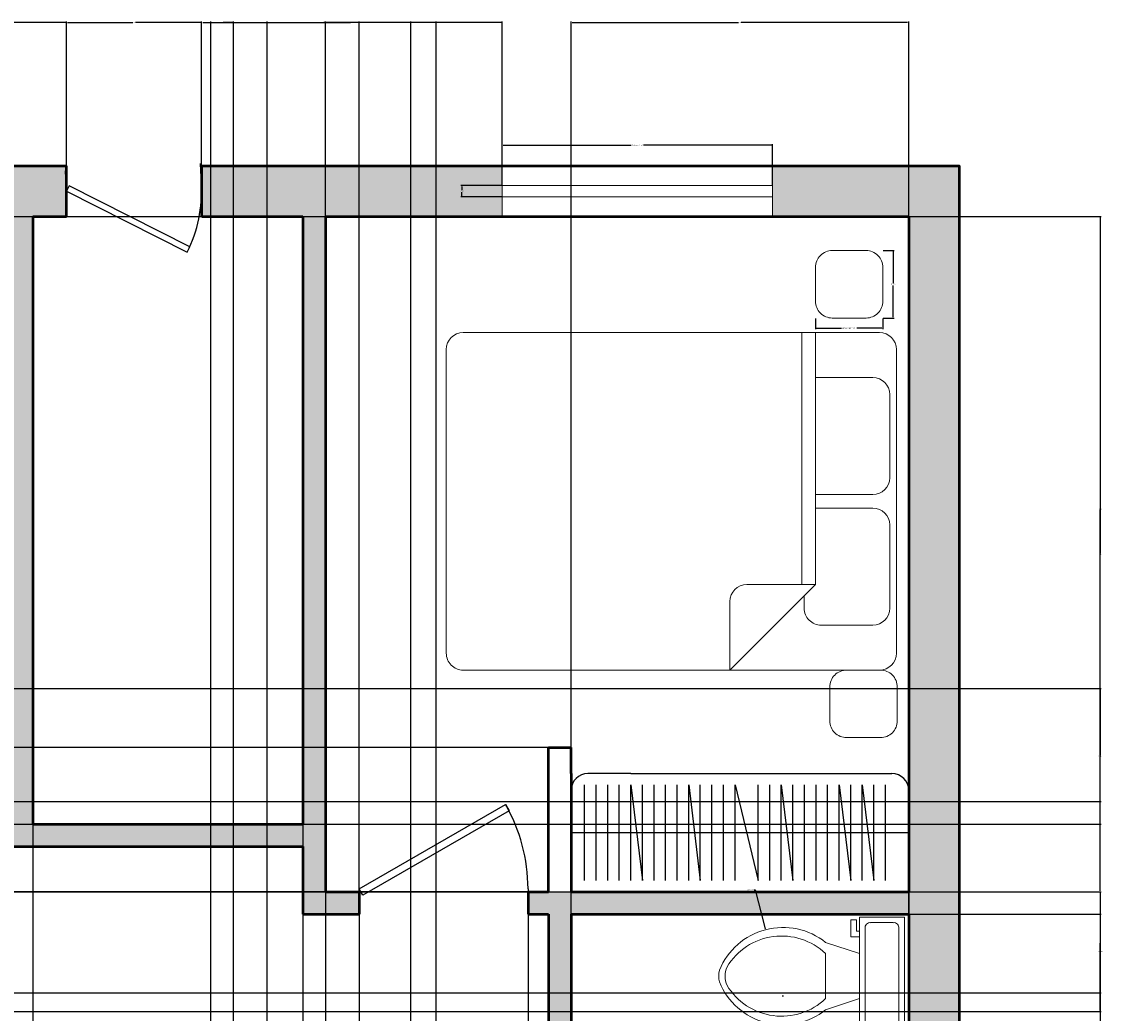
# Model space of a CAD drawing. Units: inches. Extents: x 3439 to 3988, y 1915 to 2284.
# Tile 7 of 7: x 3796 to 3988, y 2108 to 2284. Entities that reach past the tile are written whole.
import ezdxf

# ---------------------------------------------------------------- set-up
doc = ezdxf.new("R2010")
doc.units = ezdxf.units.IN
for name, color, linetype, lineweight in [('A-ANNO-DIMS', 2, 'Continuous', 18), ('A-DOOR', 3, 'Continuous', 25), ('A-FLOR-CASE', 8, 'Continuous', 25), ('A-FLOR-FIXT', 9, 'Continuous', 18), ('A-FURN', 9, 'Continuous', 18), ('A-GLAZ', 4, 'Continuous', 18), ('A-WALL', 7, 'Continuous', 50)]:
    doc.layers.add(name, color=color, linetype=linetype, lineweight=lineweight)
doc.layers.add('A-WALL-PATT', color=18, linetype='Continuous', lineweight=13, true_color=0x000000)
doc.styles.get("Standard").update_dxf_attribs({"font": 'arial.ttf'})
doc.dimstyles.get("Standard").update_dxf_attribs({"dimtxt": 0.18, "dimasz": 0.18, "dimexe": 0.18, "dimexo": 0.0625, "dimgap": 0.09, "dimtad": 0, "dimtih": 1, "dimtoh": 1, "dimdec": 4, "dimzin": 0, "dimdsep": 46, "dimtxsty": 'Standard', "dimcen": 0.09, "dimadec": 0, "dimazin": 0, "dimtfac": 1, "dimtdec": 4, "dimtofl": 0, "dimtmove": 0, "dimatfit": 3, "dimfxl": 1, "dimtolj": 1, "dimtzin": 0, "dimarcsym": 0})

# ---------------------------------------------------------------- blocks, each defined once
blk = doc.blocks.new('*U5')
for p, q in [((0, 0), (0, 6)), ((40, 0), (40, 6))]:
    blk.add_line(p, q)
blk.add_lwpolyline([(0, 0), (34.64, -20), (35.52, -18.48), (0.87, 1.52)], close=True)
blk.add_arc((0, 0), 40, 330, 0)
blk = doc.blocks.new('*U4')
for p, q in [((0, 0), (0, -6)), ((40, 0), (40, -6))]:
    blk.add_line(p, q)
blk.add_lwpolyline([(0, 0), (34.64, 20), (35.52, 18.48), (0.87, -1.52)], close=True)
blk.add_arc((0, 0), 40, 0, 30)
blk = doc.blocks.new('Toilet - top')
for p, q in [((9.5, -6), (9.5, -2)), ((-10, -8.5), (-8, -8.5)), ((-10, -9.5), (-10, -8.5)), ((-7, -9.5), (-10, -9.5)), ((-8, -8.5), (-8, -8)), ((-7, -8), (-7, -9.5)), ((-4, -8), (-6, -14)), ((4, -8), (6, -14)), ((4, -14), (-4, -14))]:
    blk.add_line(p, q)
blk.add_lwpolyline([(10.5, -8), (10.5, 0), (-10.5, 0), (-10.5, -8)], close=True)
for points in [[(8.5, -1), (-8.5, -1)], [(-9.5, -2), (-9.5, -6)], [(-8.5, -7), (8.5, -7)]]:
    blk.add_lwpolyline(points)
for centre, radius, start, end in [((-8.62, -1.88), 0.884, 81.8699, 188.1301), ((8.62, -1.88), 0.884, 351.8699, 98.1301), ((-8.62, -6.12), 0.884, 171.8699, 278.1301), ((8.62, -6.12), 0.884, 261.8699, 8.1301), ((3.52, -21.58), 12.17, 141.4691, 247.9714), ((4.2, -21.82), 11.33, 136.3677, 238.9468), ((-3.52, -21.58), 12.17, 292.0284, 38.5307), ((-4.2, -21.82), 11.33, 301.053, 43.6321), ((0, -27.88), 4, 245.7318, 294.2682), ((0, -29), 4, 254.8605, 285.1395)]:
    blk.add_arc(centre, radius, start, end)
blk = doc.blocks.new('Bed - Queen')
for p, q in [((3, 0), (56.99999, 0)), ((10.99999, -1.2), (25.79998, -1.2)), ((34.19999, -1.2), (48.99999, -1.2)), ((0, -77.00003), (0, -3)), ((59.99999, -3), (59.99999, -77.00003)), ((7.99999, -14.4), (7.99999, -4.2)), ((28.79998, -4.2), (28.79998, -14.4)), ((31.19999, -14.4), (31.19999, -4.2)), ((51.99999, -4.2), (51.99999, -13.4)), ((0, -14.4), (44.8, -14.4)), ((59.99999, -29.6), (44.8, -14.4)), ((44.8, -14.4), (44.8, -26.6)), ((44.8, -16.8), (0, -16.8)), ((48.99999, -16.4), (46.79936, -16.4)), ((47.8, -29.6), (59.99999, -29.6)), ((56.99999, -80.00003), (3, -80.00003))]:
    blk.add_line(p, q)
for centre, start, end in [((3, -3), 90, 180), ((56.99999, -3), 0, 90), ((10.99999, -4.2), 90, 180), ((25.79998, -4.2), 0, 90), ((34.19999, -4.2), 90, 180), ((48.99999, -4.2), 0, 90), ((48.99999, -13.4), 270, 0), ((47.8, -26.6), 180, 270), ((3, -77.00003), 180, 270), ((56.99999, -77.00003), 270, 0)]:
    blk.add_arc(centre, 3, start, end)
blk = doc.blocks.new('WINDOW-GLASS-48IN')
for p, q in [((0, 2), (48, 2)), ((0, 0), (48, 0))]:
    blk.add_line(p, q)
blk = doc.blocks.new('NIGHTSTAND-12IN-RADIUS')
blk.add_lwpolyline([(3, 0), (9, 0, 0.414214), (12, 3), (12, 9, 0.414214), (9, 12), (3, 12, 0.414214), (0, 9), (0, 3, 0.414214)], format="xyb", close=True)
blk = doc.blocks.new('*D19')
at = {"layer": 'A-ANNO-DIMS', "color": 0, "lineweight": -2, "transparency": 16777216}
for p, q in [((3881.36, 2254.92), (3881.36, 2262.24)), ((3881.54, 2262.06), (3904.24, 2262.06)), ((3929.18, 2262.06), (3906.47, 2262.06)), ((3929.36, 2254.92), (3929.36, 2262.24))]:
    blk.add_line(p, q, dxfattribs=at)
at = {"layer": 'A-ANNO-DIMS', "color": 0, "transparency": 16777216}
for points in [[(3881.54, 2262.09), (3881.54, 2262.03), (3881.36, 2262.06)], [(3929.18, 2262.09), (3929.18, 2262.03), (3929.36, 2262.06)]]:
    blk.add_solid(points, dxfattribs=at)
at = {"layer": 'Defpoints', "color": 0, "transparency": 16777216}
for p in [(3929.36, 2262.06), (3881.36, 2254.86), (3929.36, 2254.86)]:
    blk.add_point(p, dxfattribs=at)
at = {"layer": 'A-ANNO-DIMS', "color": 0, "transparency": 16777216, "insert": (3905.36, 2262.06), "char_height": 0.18, "attachment_point": 5}
blk.add_mtext('\\A1;WINDOW 48 TYP.', dxfattribs=at)
blk = doc.blocks.new('*D20')
at = {"layer": 'A-ANNO-DIMS', "color": 0, "lineweight": -2, "transparency": 16777216}
for p, q in [((3881.29, 2254.86), (3873.98, 2254.86)), ((3874.16, 2254.68), (3874.16, 2254.04)), ((3874.16, 2253.04), (3874.16, 2253.68)), ((3881.29, 2252.86), (3873.98, 2252.86))]:
    blk.add_line(p, q, dxfattribs=at)
at = {"layer": 'A-ANNO-DIMS', "color": 0, "transparency": 16777216}
for points in [[(3874.13, 2254.68), (3874.19, 2254.68), (3874.16, 2254.86)], [(3874.13, 2253.04), (3874.19, 2253.04), (3874.16, 2252.86)]]:
    blk.add_solid(points, dxfattribs=at)
at = {"layer": 'Defpoints', "color": 0, "transparency": 16777216}
for p in [(3874.16, 2254.86), (3881.36, 2254.86), (3881.36, 2252.86)]:
    blk.add_point(p, dxfattribs=at)
at = {"layer": 'A-ANNO-DIMS', "color": 0, "transparency": 16777216, "insert": (3874.16, 2253.86), "char_height": 0.18, "attachment_point": 5}
blk.add_mtext('\\A1;2 TYP.', dxfattribs=at)
blk = doc.blocks.new('*D27')
at = {"layer": 'A-ANNO-DIMS', "color": 0, "lineweight": -2, "transparency": 16777216}
for p, q in [((3937, 2231.25), (3937, 2229.33)), ((3949, 2231.25), (3949, 2229.33)), ((3937.18, 2229.51), (3941.63, 2229.51)), ((3948.82, 2229.51), (3944.38, 2229.51))]:
    blk.add_line(p, q, dxfattribs=at)
at = {"layer": 'A-ANNO-DIMS', "color": 0, "transparency": 16777216}
for points in [[(3937.18, 2229.54), (3937.18, 2229.48), (3937, 2229.51)], [(3948.82, 2229.54), (3948.82, 2229.48), (3949, 2229.51)]]:
    blk.add_solid(points, dxfattribs=at)
at = {"layer": 'Defpoints', "color": 0, "transparency": 16777216}
for p in [(3937, 2231.31), (3949, 2231.31), (3949, 2229.51)]:
    blk.add_point(p, dxfattribs=at)
at = {"layer": 'A-ANNO-DIMS', "color": 0, "transparency": 16777216, "insert": (3943, 2229.51), "char_height": 0.18, "attachment_point": 5}
blk.add_mtext('\\A1;NIGHTSTAND 12 TYP.', dxfattribs=at)
blk = doc.blocks.new('*D28')
at = {"layer": 'A-ANNO-DIMS', "color": 0, "lineweight": -2, "transparency": 16777216}
for p, q in [((3949.07, 2243.31), (3950.98, 2243.31)), ((3950.8, 2243.13), (3950.8, 2237.49)), ((3950.8, 2231.49), (3950.8, 2237.13)), ((3949.07, 2231.31), (3950.98, 2231.31))]:
    blk.add_line(p, q, dxfattribs=at)
at = {"layer": 'A-ANNO-DIMS', "color": 0, "transparency": 16777216}
for points in [[(3950.77, 2243.13), (3950.83, 2243.13), (3950.8, 2243.31)], [(3950.77, 2231.49), (3950.83, 2231.49), (3950.8, 2231.31)]]:
    blk.add_solid(points, dxfattribs=at)
at = {"layer": 'Defpoints', "color": 0, "transparency": 16777216}
for p in [(3949, 2243.31), (3950.8, 2243.31), (3949, 2231.31)]:
    blk.add_point(p, dxfattribs=at)
at = {"layer": 'A-ANNO-DIMS', "color": 0, "transparency": 16777216, "insert": (3950.8, 2237.31), "char_height": 0.18, "attachment_point": 5}
blk.add_mtext('\\A1;12 TYP.', dxfattribs=at)
blk = doc.blocks.new('*D50')
at = {"layer": 'A-ANNO-DIMS', "color": 0, "lineweight": -2, "transparency": 16777216}
for p, q in [((3797.93, 2249.3), (3797.93, 1915.13)), ((3845.93, 2249.3), (3845.93, 1915.13)), ((3798.11, 1915.31), (3821.71, 1915.31)), ((3845.75, 1915.31), (3822.15, 1915.31))]:
    blk.add_line(p, q, dxfattribs=at)
at = {"layer": 'A-ANNO-DIMS', "color": 0, "transparency": 16777216}
for points in [[(3798.11, 1915.34), (3798.11, 1915.28), (3797.93, 1915.31)], [(3845.75, 1915.34), (3845.75, 1915.28), (3845.93, 1915.31)]]:
    blk.add_solid(points, dxfattribs=at)
at = {"layer": 'Defpoints', "color": 0, "transparency": 16777216}
for p in [(3797.93, 2249.36), (3845.93, 2249.36), (3845.93, 1915.31)]:
    blk.add_point(p, dxfattribs=at)
at = {"layer": 'A-ANNO-DIMS', "color": 0, "transparency": 16777216, "insert": (3821.93, 1915.31), "char_height": 0.18, "attachment_point": 5}
blk.add_mtext('\\A1;48', dxfattribs=at)
blk = doc.blocks.new('*D51')
at = {"layer": 'A-ANNO-DIMS', "color": 0, "lineweight": -2, "transparency": 16777216}
for p, q in [((3849.93, 2249.3), (3849.93, 1915.13)), ((3953.58, 2249.3), (3953.58, 1915.13)), ((3850.11, 1915.31), (3901.3, 1915.31)), ((3953.4, 1915.31), (3902.21, 1915.31))]:
    blk.add_line(p, q, dxfattribs=at)
at = {"layer": 'A-ANNO-DIMS', "color": 0, "transparency": 16777216}
for points in [[(3850.11, 1915.34), (3850.11, 1915.28), (3849.93, 1915.31)], [(3953.4, 1915.34), (3953.4, 1915.28), (3953.58, 1915.31)]]:
    blk.add_solid(points, dxfattribs=at)
at = {"layer": 'Defpoints', "color": 0, "transparency": 16777216}
for p in [(3849.93, 2249.36), (3953.58, 2249.36), (3953.58, 1915.31)]:
    blk.add_point(p, dxfattribs=at)
at = {"layer": 'A-ANNO-DIMS', "color": 0, "transparency": 16777216, "insert": (3901.76, 1915.31), "char_height": 0.18, "attachment_point": 5}
blk.add_mtext('\\A1;103.65', dxfattribs=at)
blk = doc.blocks.new('*D58')
at = {"layer": 'A-ANNO-DIMS', "color": 0, "lineweight": -2, "transparency": 16777216}
for p, q in [((3953.64, 2249.36), (3987.81, 2249.36)), ((3987.63, 2249.18), (3987.63, 2189.54)), ((3987.63, 2129.54), (3987.63, 2189.18)), ((3953.64, 2129.36), (3987.81, 2129.36))]:
    blk.add_line(p, q, dxfattribs=at)
at = {"layer": 'A-ANNO-DIMS', "color": 0, "transparency": 16777216}
for points in [[(3987.6, 2249.18), (3987.66, 2249.18), (3987.63, 2249.36)], [(3987.6, 2129.54), (3987.66, 2129.54), (3987.63, 2129.36)]]:
    blk.add_solid(points, dxfattribs=at)
at = {"layer": 'Defpoints', "color": 0, "transparency": 16777216}
for p in [(3953.58, 2249.36), (3987.63, 2249.36), (3953.58, 2129.36)]:
    blk.add_point(p, dxfattribs=at)
at = {"layer": 'A-ANNO-DIMS', "color": 0, "transparency": 16777216, "insert": (3987.63, 2189.36), "char_height": 0.18, "attachment_point": 5}
blk.add_mtext('\\A1;120', dxfattribs=at)
blk = doc.blocks.new('*D59')
at = {"layer": 'A-ANNO-DIMS', "color": 0, "lineweight": -2, "transparency": 16777216}
for p, q in [((3953.64, 2125.36), (3987.81, 2125.36)), ((3987.63, 2125.18), (3987.63, 2095.54)), ((3987.63, 2065.54), (3987.63, 2095.18)), ((3953.64, 2065.36), (3987.81, 2065.36))]:
    blk.add_line(p, q, dxfattribs=at)
at = {"layer": 'A-ANNO-DIMS', "color": 0, "transparency": 16777216}
for points in [[(3987.6, 2125.18), (3987.66, 2125.18), (3987.63, 2125.36)], [(3987.6, 2065.54), (3987.66, 2065.54), (3987.63, 2065.36)]]:
    blk.add_solid(points, dxfattribs=at)
at = {"layer": 'Defpoints', "color": 0, "transparency": 16777216}
for p in [(3953.58, 2125.36), (3987.63, 2125.36), (3953.58, 2065.36)]:
    blk.add_point(p, dxfattribs=at)
at = {"layer": 'A-ANNO-DIMS', "color": 0, "transparency": 16777216, "insert": (3987.63, 2095.36), "char_height": 0.18, "attachment_point": 5}
blk.add_mtext('\\A1;60', dxfattribs=at)
blk = doc.blocks.new('*D63')
at = {"layer": 'A-ANNO-DIMS', "color": 0, "lineweight": -2, "transparency": 16777216}
for p, q in [((3893.58, 2065.42), (3893.58, 2284)), ((3893.76, 2283.82), (3923.36, 2283.82)), ((3953.4, 2283.82), (3923.8, 2283.82)), ((3953.58, 2065.42), (3953.58, 2284))]:
    blk.add_line(p, q, dxfattribs=at)
at = {"layer": 'A-ANNO-DIMS', "color": 0, "transparency": 16777216}
for points in [[(3893.76, 2283.85), (3893.76, 2283.79), (3893.58, 2283.82)], [(3953.4, 2283.85), (3953.4, 2283.79), (3953.58, 2283.82)]]:
    blk.add_solid(points, dxfattribs=at)
at = {"layer": 'Defpoints', "color": 0, "transparency": 16777216}
for p in [(3953.58, 2283.82), (3893.58, 2065.36), (3953.58, 2065.36)]:
    blk.add_point(p, dxfattribs=at)
at = {"layer": 'A-ANNO-DIMS', "color": 0, "transparency": 16777216, "insert": (3923.58, 2283.82), "char_height": 0.18, "attachment_point": 5}
blk.add_mtext('\\A1;60', dxfattribs=at)
blk = doc.blocks.new('*D64')
at = {"layer": 'A-ANNO-DIMS', "color": 0, "lineweight": -2, "transparency": 16777216}
for p, q in [((3593.64, 2249.36), (3987.81, 2249.36)), ((3987.63, 2249.18), (3987.63, 2197.54)), ((3987.63, 2145.54), (3987.63, 2197.18)), ((3593.64, 2145.36), (3987.81, 2145.36))]:
    blk.add_line(p, q, dxfattribs=at)
at = {"layer": 'A-ANNO-DIMS', "color": 0, "transparency": 16777216}
for points in [[(3987.6, 2249.18), (3987.66, 2249.18), (3987.63, 2249.36)], [(3987.6, 2145.54), (3987.66, 2145.54), (3987.63, 2145.36)]]:
    blk.add_solid(points, dxfattribs=at)
at = {"layer": 'Defpoints', "color": 0, "transparency": 16777216}
for p in [(3593.58, 2249.36), (3987.63, 2249.36), (3593.58, 2145.36)]:
    blk.add_point(p, dxfattribs=at)
at = {"layer": 'A-ANNO-DIMS', "color": 0, "transparency": 16777216, "insert": (3987.63, 2197.36), "char_height": 0.18, "attachment_point": 5}
blk.add_mtext('\\A1;104', dxfattribs=at)
blk = doc.blocks.new('*D65')
at = {"layer": 'A-ANNO-DIMS', "color": 0, "lineweight": -2, "transparency": 16777216}
for p, q in [((3797.99, 2249.36), (3987.81, 2249.36)), ((3987.63, 2249.18), (3987.63, 2195.54)), ((3987.63, 2141.54), (3987.63, 2195.18)), ((3797.99, 2141.36), (3987.81, 2141.36))]:
    blk.add_line(p, q, dxfattribs=at)
at = {"layer": 'A-ANNO-DIMS', "color": 0, "transparency": 16777216}
for points in [[(3987.6, 2249.18), (3987.66, 2249.18), (3987.63, 2249.36)], [(3987.6, 2141.54), (3987.66, 2141.54), (3987.63, 2141.36)]]:
    blk.add_solid(points, dxfattribs=at)
at = {"layer": 'Defpoints', "color": 0, "transparency": 16777216}
for p in [(3797.93, 2249.36), (3987.63, 2249.36), (3797.93, 2141.36)]:
    blk.add_point(p, dxfattribs=at)
at = {"layer": 'A-ANNO-DIMS', "color": 0, "transparency": 16777216, "insert": (3987.63, 2195.36), "char_height": 0.18, "attachment_point": 5}
blk.add_mtext('\\A1;108', dxfattribs=at)
blk = doc.blocks.new('*D69')
at = {"layer": 'A-ANNO-DIMS', "color": 0, "lineweight": -2, "transparency": 16777216}
for p, q in [((3739.41, 2258.42), (3739.41, 2284)), ((3739.59, 2283.82), (3771.27, 2283.82)), ((3803.75, 2283.82), (3772.06, 2283.82)), ((3803.93, 2258.42), (3803.93, 2284))]:
    blk.add_line(p, q, dxfattribs=at)
at = {"layer": 'A-ANNO-DIMS', "color": 0, "transparency": 16777216}
for points in [[(3739.59, 2283.85), (3739.59, 2283.79), (3739.41, 2283.82)], [(3803.75, 2283.85), (3803.75, 2283.79), (3803.93, 2283.82)]]:
    blk.add_solid(points, dxfattribs=at)
at = {"layer": 'Defpoints', "color": 0, "transparency": 16777216}
for p in [(3803.93, 2283.82), (3739.41, 2258.36), (3803.93, 2258.36)]:
    blk.add_point(p, dxfattribs=at)
at = {"layer": 'A-ANNO-DIMS', "color": 0, "transparency": 16777216, "insert": (3771.67, 2283.82), "char_height": 0.18, "attachment_point": 5}
blk.add_mtext('\\A1;64.53', dxfattribs=at)
blk = doc.blocks.new('*D70')
at = {"layer": 'A-ANNO-DIMS', "color": 0, "lineweight": -2, "transparency": 16777216}
for p, q in [((3803.93, 2258.42), (3803.93, 2284)), ((3804.11, 2283.82), (3815.71, 2283.82)), ((3827.75, 2283.82), (3816.15, 2283.82)), ((3827.93, 2258.42), (3827.93, 2284))]:
    blk.add_line(p, q, dxfattribs=at)
at = {"layer": 'A-ANNO-DIMS', "color": 0, "transparency": 16777216}
for points in [[(3804.11, 2283.85), (3804.11, 2283.79), (3803.93, 2283.82)], [(3827.75, 2283.85), (3827.75, 2283.79), (3827.93, 2283.82)]]:
    blk.add_solid(points, dxfattribs=at)
at = {"layer": 'Defpoints', "color": 0, "transparency": 16777216}
for p in [(3827.93, 2283.82), (3803.93, 2258.36), (3827.93, 2258.36)]:
    blk.add_point(p, dxfattribs=at)
at = {"layer": 'A-ANNO-DIMS', "color": 0, "transparency": 16777216, "insert": (3815.93, 2283.82), "char_height": 0.18, "attachment_point": 5}
blk.add_mtext('\\A1;24', dxfattribs=at)
blk = doc.blocks.new('*D71')
at = {"layer": 'A-ANNO-DIMS', "color": 0, "lineweight": -2, "transparency": 16777216}
for p, q in [((3827.93, 2258.42), (3827.93, 2284)), ((3828.11, 2283.82), (3854.25, 2283.82)), ((3881.18, 2283.82), (3855.04, 2283.82)), ((3881.36, 2258.42), (3881.36, 2284))]:
    blk.add_line(p, q, dxfattribs=at)
at = {"layer": 'A-ANNO-DIMS', "color": 0, "transparency": 16777216}
for points in [[(3828.11, 2283.85), (3828.11, 2283.79), (3827.93, 2283.82)], [(3881.18, 2283.85), (3881.18, 2283.79), (3881.36, 2283.82)]]:
    blk.add_solid(points, dxfattribs=at)
at = {"layer": 'Defpoints', "color": 0, "transparency": 16777216}
for p in [(3881.36, 2283.82), (3827.93, 2258.36), (3881.36, 2258.36)]:
    blk.add_point(p, dxfattribs=at)
at = {"layer": 'A-ANNO-DIMS', "color": 0, "transparency": 16777216, "insert": (3854.64, 2283.82), "char_height": 0.18, "attachment_point": 5}
blk.add_mtext('\\A1;53.42', dxfattribs=at)
blk = doc.blocks.new('*D76')
at = {"layer": 'A-ANNO-DIMS', "color": 0, "lineweight": -2, "transparency": 16777216}
for p, q in [((3833.58, 1949.42), (3833.58, 2284)), ((3833.76, 2283.82), (3849.01, 2283.82)), ((3864.9, 2283.82), (3849.66, 2283.82)), ((3865.08, 1949.42), (3865.08, 2284))]:
    blk.add_line(p, q, dxfattribs=at)
at = {"layer": 'A-ANNO-DIMS', "color": 0, "transparency": 16777216}
for points in [[(3833.76, 2283.85), (3833.76, 2283.79), (3833.58, 2283.82)], [(3864.9, 2283.85), (3864.9, 2283.79), (3865.08, 2283.82)]]:
    blk.add_solid(points, dxfattribs=at)
at = {"layer": 'Defpoints', "color": 0, "transparency": 16777216}
for p in [(3865.08, 2283.82), (3833.58, 1949.36), (3865.08, 1949.36)]:
    blk.add_point(p, dxfattribs=at)
at = {"layer": 'A-ANNO-DIMS', "color": 0, "transparency": 16777216, "insert": (3849.33, 2283.82), "char_height": 0.18, "attachment_point": 5}
blk.add_mtext('\\A1;31.5', dxfattribs=at)
blk = doc.blocks.new('*D77')
at = {"layer": 'A-ANNO-DIMS', "color": 0, "lineweight": -2, "transparency": 16777216}
for p, q in [((3473.64, 2129.36), (3987.81, 2129.36)), ((3987.63, 2129.18), (3987.63, 2118.9)), ((3987.63, 2108.25), (3987.63, 2118.53)), ((3473.64, 2108.07), (3987.81, 2108.07))]:
    blk.add_line(p, q, dxfattribs=at)
at = {"layer": 'A-ANNO-DIMS', "color": 0, "transparency": 16777216}
for points in [[(3987.6, 2129.18), (3987.66, 2129.18), (3987.63, 2129.36)], [(3987.6, 2108.25), (3987.66, 2108.25), (3987.63, 2108.07)]]:
    blk.add_solid(points, dxfattribs=at)
at = {"layer": 'Defpoints', "color": 0, "transparency": 16777216}
for p in [(3473.58, 2129.36), (3987.63, 2129.36), (3473.58, 2108.07)]:
    blk.add_point(p, dxfattribs=at)
at = {"layer": 'A-ANNO-DIMS', "color": 0, "transparency": 16777216, "insert": (3987.63, 2118.71), "char_height": 0.18, "attachment_point": 5}
blk.add_mtext('\\A1;21.295', dxfattribs=at)
blk = doc.blocks.new('*D82')
at = {"layer": 'A-ANNO-DIMS', "color": 0, "lineweight": -2, "transparency": 16777216}
for p, q in [((3537.64, 2129.36), (3987.81, 2129.36)), ((3987.63, 2129.18), (3987.63, 2120.54)), ((3987.63, 2111.54), (3987.63, 2120.18)), ((3537.64, 2111.36), (3987.81, 2111.36))]:
    blk.add_line(p, q, dxfattribs=at)
at = {"layer": 'A-ANNO-DIMS', "color": 0, "transparency": 16777216}
for points in [[(3987.6, 2129.18), (3987.66, 2129.18), (3987.63, 2129.36)], [(3987.6, 2111.54), (3987.66, 2111.54), (3987.63, 2111.36)]]:
    blk.add_solid(points, dxfattribs=at)
at = {"layer": 'Defpoints', "color": 0, "transparency": 16777216}
for p in [(3537.58, 2129.36), (3987.63, 2129.36), (3537.58, 2111.36)]:
    blk.add_point(p, dxfattribs=at)
at = {"layer": 'A-ANNO-DIMS', "color": 0, "transparency": 16777216, "insert": (3987.63, 2120.36), "char_height": 0.18, "attachment_point": 5}
blk.add_mtext('\\A1;18', dxfattribs=at)
blk = doc.blocks.new('*D83')
at = {"layer": 'A-ANNO-DIMS', "color": 0, "lineweight": -2, "transparency": 16777216}
for p, q in [((3537.64, 2111.36), (3987.81, 2111.36)), ((3987.63, 2111.18), (3987.63, 2099.54)), ((3987.63, 2087.54), (3987.63, 2099.18)), ((3537.64, 2087.36), (3987.81, 2087.36))]:
    blk.add_line(p, q, dxfattribs=at)
at = {"layer": 'A-ANNO-DIMS', "color": 0, "transparency": 16777216}
for points in [[(3987.6, 2111.18), (3987.66, 2111.18), (3987.63, 2111.36)], [(3987.6, 2087.54), (3987.66, 2087.54), (3987.63, 2087.36)]]:
    blk.add_solid(points, dxfattribs=at)
at = {"layer": 'Defpoints', "color": 0, "transparency": 16777216}
for p in [(3537.58, 2111.36), (3987.63, 2111.36), (3537.58, 2087.36)]:
    blk.add_point(p, dxfattribs=at)
at = {"layer": 'A-ANNO-DIMS', "color": 0, "transparency": 16777216, "insert": (3987.63, 2099.36), "char_height": 0.18, "attachment_point": 5}
blk.add_mtext('\\A1;24', dxfattribs=at)
blk = doc.blocks.new('*D84')
at = {"layer": 'A-ANNO-DIMS', "color": 0, "lineweight": -2, "transparency": 16777216}
for p, q in [((3849.93, 2129.42), (3849.93, 2284)), ((3850.11, 2283.82), (3852.78, 2283.82)), ((3855.75, 2283.82), (3853.08, 2283.82)), ((3855.93, 2129.42), (3855.93, 2284))]:
    blk.add_line(p, q, dxfattribs=at)
at = {"layer": 'A-ANNO-DIMS', "color": 0, "transparency": 16777216}
for points in [[(3850.11, 2283.85), (3850.11, 2283.79), (3849.93, 2283.82)], [(3855.75, 2283.85), (3855.75, 2283.79), (3855.93, 2283.82)]]:
    blk.add_solid(points, dxfattribs=at)
at = {"layer": 'Defpoints', "color": 0, "transparency": 16777216}
for p in [(3855.93, 2283.82), (3849.93, 2129.36), (3855.93, 2129.36)]:
    blk.add_point(p, dxfattribs=at)
at = {"layer": 'A-ANNO-DIMS', "color": 0, "transparency": 16777216, "insert": (3852.93, 2283.82), "char_height": 0.18, "attachment_point": 5}
blk.add_mtext('\\A1;6', dxfattribs=at)
blk = doc.blocks.new('*D85')
at = {"layer": 'A-ANNO-DIMS', "color": 0, "lineweight": -2, "transparency": 16777216}
for p, q in [((3855.93, 2125.3), (3855.93, 1915.13)), ((3885.93, 2125.3), (3885.93, 1915.13)), ((3856.11, 1915.31), (3870.71, 1915.31)), ((3885.75, 1915.31), (3871.15, 1915.31))]:
    blk.add_line(p, q, dxfattribs=at)
at = {"layer": 'A-ANNO-DIMS', "color": 0, "transparency": 16777216}
for points in [[(3856.11, 1915.34), (3856.11, 1915.28), (3855.93, 1915.31)], [(3885.75, 1915.34), (3885.75, 1915.28), (3885.93, 1915.31)]]:
    blk.add_solid(points, dxfattribs=at)
at = {"layer": 'Defpoints', "color": 0, "transparency": 16777216}
for p in [(3855.93, 2125.36), (3885.93, 2125.36), (3885.93, 1915.31)]:
    blk.add_point(p, dxfattribs=at)
at = {"layer": 'A-ANNO-DIMS', "color": 0, "transparency": 16777216, "insert": (3870.93, 1915.31), "char_height": 0.18, "attachment_point": 5}
blk.add_mtext('\\A1;30', dxfattribs=at)
blk = doc.blocks.new('*D87')
at = {"layer": 'A-ANNO-DIMS', "color": 0, "lineweight": -2, "transparency": 16777216}
for p, q in [((3839.58, 2065.42), (3839.58, 2284)), ((3839.76, 2283.82), (3854.36, 2283.82)), ((3869.4, 2283.82), (3854.8, 2283.82)), ((3869.58, 2065.42), (3869.58, 2284))]:
    blk.add_line(p, q, dxfattribs=at)
at = {"layer": 'A-ANNO-DIMS', "color": 0, "transparency": 16777216}
for points in [[(3839.76, 2283.85), (3839.76, 2283.79), (3839.58, 2283.82)], [(3869.4, 2283.85), (3869.4, 2283.79), (3869.58, 2283.82)]]:
    blk.add_solid(points, dxfattribs=at)
at = {"layer": 'Defpoints', "color": 0, "transparency": 16777216}
for p in [(3869.58, 2283.82), (3839.58, 2065.36), (3869.58, 2065.36)]:
    blk.add_point(p, dxfattribs=at)
at = {"layer": 'A-ANNO-DIMS', "color": 0, "transparency": 16777216, "insert": (3854.58, 2283.82), "char_height": 0.18, "attachment_point": 5}
blk.add_mtext('\\A1;30', dxfattribs=at)
blk = doc.blocks.new('*D93')
at = {"layer": 'A-ANNO-DIMS', "color": 0, "lineweight": -2, "transparency": 16777216}
for p, q in [((3829.58, 2065.42), (3829.58, 2284)), ((3829.76, 2283.82), (3831.43, 2283.82)), ((3833.4, 2283.82), (3831.73, 2283.82)), ((3833.58, 2061.42), (3833.58, 2284))]:
    blk.add_line(p, q, dxfattribs=at)
at = {"layer": 'A-ANNO-DIMS', "color": 0, "transparency": 16777216}
for points in [[(3829.76, 2283.85), (3829.76, 2283.79), (3829.58, 2283.82)], [(3833.4, 2283.85), (3833.4, 2283.79), (3833.58, 2283.82)]]:
    blk.add_solid(points, dxfattribs=at)
at = {"layer": 'Defpoints', "color": 0, "transparency": 16777216}
for p in [(3833.58, 2283.82), (3829.58, 2065.36), (3833.58, 2061.36)]:
    blk.add_point(p, dxfattribs=at)
at = {"layer": 'A-ANNO-DIMS', "color": 0, "transparency": 16777216, "insert": (3831.58, 2283.82), "char_height": 0.18, "attachment_point": 5}
blk.add_mtext('\\A1;4', dxfattribs=at)
blk = doc.blocks.new('*D95')
at = {"layer": 'A-ANNO-DIMS', "color": 0, "lineweight": -2, "transparency": 16777216}
for p, q in [((3729.47, 2165.5), (3987.81, 2165.5)), ((3987.63, 2165.32), (3987.63, 2153.61)), ((3987.63, 2141.54), (3987.63, 2153.25)), ((3729.47, 2141.36), (3987.81, 2141.36))]:
    blk.add_line(p, q, dxfattribs=at)
at = {"layer": 'A-ANNO-DIMS', "color": 0, "transparency": 16777216}
for points in [[(3987.6, 2165.32), (3987.66, 2165.32), (3987.63, 2165.5)], [(3987.6, 2141.54), (3987.66, 2141.54), (3987.63, 2141.36)]]:
    blk.add_solid(points, dxfattribs=at)
at = {"layer": 'Defpoints', "color": 0, "transparency": 16777216}
for p in [(3729.41, 2165.5), (3987.63, 2165.5), (3729.41, 2141.36)]:
    blk.add_point(p, dxfattribs=at)
at = {"layer": 'A-ANNO-DIMS', "color": 0, "transparency": 16777216, "insert": (3987.63, 2153.43), "char_height": 0.18, "attachment_point": 5}
blk.add_mtext('\\A1;24.14', dxfattribs=at)
blk = doc.blocks.new('*D98')
at = {"layer": 'A-ANNO-DIMS', "color": 0, "lineweight": -2, "transparency": 16777216}
for p, q in [((3889.52, 2154.99), (3439.35, 2154.99)), ((3439.53, 2154.81), (3439.53, 2142.36)), ((3439.53, 2129.54), (3439.53, 2141.99)), ((3889.52, 2129.36), (3439.35, 2129.36))]:
    blk.add_line(p, q, dxfattribs=at)
at = {"layer": 'A-ANNO-DIMS', "color": 0, "transparency": 16777216}
for points in [[(3439.5, 2154.81), (3439.56, 2154.81), (3439.53, 2154.99)], [(3439.5, 2129.54), (3439.56, 2129.54), (3439.53, 2129.36)]]:
    blk.add_solid(points, dxfattribs=at)
at = {"layer": 'Defpoints', "color": 0, "transparency": 16777216}
for p in [(3889.58, 2154.99), (3439.53, 2129.36), (3889.58, 2129.36)]:
    blk.add_point(p, dxfattribs=at)
at = {"layer": 'A-ANNO-DIMS', "color": 0, "transparency": 16777216, "insert": (3439.53, 2142.18), "char_height": 0.18, "attachment_point": 5}
blk.add_mtext('\\A1;25.63', dxfattribs=at)
blk = doc.blocks.new('*D103')
at = {"layer": 'A-ANNO-DIMS', "color": 0, "lineweight": -2, "transparency": 16777216}
for p, q in [((3926.12, 2129.67), (3926.3, 2129.67)), ((3926.3, 2129.67), (3928.1, 2122.78)), ((3931.24, 2110.74), (3931.24, 2110.92)), ((3931.15, 2110.83), (3931.33, 2110.83))]:
    blk.add_line(p, q, dxfattribs=at)
at = {"layer": 'A-ANNO-DIMS', "color": 0, "transparency": 16777216}
blk.add_solid([(3928.13, 2122.79), (3928.08, 2122.77), (3928.15, 2122.6)], dxfattribs=at)
at = {"layer": 'Defpoints', "color": 0, "transparency": 16777216}
for p in [(3928.15, 2122.6), (3931.24, 2110.83)]:
    blk.add_point(p, dxfattribs=at)
at = {"layer": 'A-ANNO-DIMS', "color": 0, "transparency": 16777216, "insert": (3925.44, 2129.67), "char_height": 0.18, "attachment_point": 5}
blk.add_mtext('\\A1;6X R12.17', dxfattribs=at)

msp = doc.modelspace()

# ---------------------------------------------------------------- hatches: boundary and pattern name
at = {"layer": 'A-WALL-PATT'}
h = msp.add_hatch(color=256, dxfattribs=at)
h.dxf.hatch_style = 1
h.paths.add_polyline_path([(3803.9319, 2258.3617), (3739.4053, 2258.3617), (3739.4053, 2249.3617), (3793.9319, 2249.3617), (3793.9319, 2137.3617), (3845.9319, 2137.3617), (3845.9319, 2125.3617), (3855.9319, 2125.3617), (3855.9319, 2129.3617), (3849.9319, 2129.3617), (3849.9319, 2249.3617), (3881.3564, 2249.3617), (3881.3564, 2258.3617), (3827.9319, 2258.3617), (3827.9319, 2249.3617), (3845.9319, 2249.3617), (3845.9319, 2141.3617), (3797.9319, 2141.3617), (3797.9319, 2249.3617), (3803.9319, 2249.3617)])
h = msp.add_hatch(color=256, dxfattribs=at)
h.dxf.hatch_style = 1
h.paths.add_polyline_path([(3962.5815, 2258.3617), (3929.3564, 2258.3617), (3929.3564, 2249.3617), (3953.5815, 2249.3617), (3953.5815, 2129.3617), (3885.9319, 2129.3617), (3885.9319, 2125.3617), (3889.5815, 2125.3617), (3889.5815, 2095.3617), (3893.5815, 2095.3617), (3893.5815, 2125.3617), (3953.5815, 2125.3617), (3953.5815, 2065.3617), (3893.5815, 2065.3617), (3893.5815, 2071.3617), (3889.5815, 2071.3617), (3889.5815, 2065.3617), (3869.5815, 2065.3617), (3869.5815, 2061.3617), (3953.5815, 2061.3617), (3953.5815, 1949.3617), (3913.0815, 1949.3617), (3913.0815, 1940.3617), (3962.5815, 1940.3617)])

# ---------------------------------------------------------------- linework, layer by layer
at = {"layer": 'A-FLOR-CASE'}
for p, q in [((3904.206, 2150.3617), (3896.5815, 2150.3617)), ((3904.206, 2150.3617), (3950.5815, 2150.3617)), ((3904.206, 2150.3617), (3950.5815, 2150.3617)), ((3953.5815, 2150.3617), (3953.5815, 2129.3617)), ((3895.9789, 2131.3617), (3895.9789, 2148.3617)), ((3895.9789, 2131.3617), (3895.9789, 2148.3617)), ((3898.0357, 2131.3617), (3898.0357, 2148.3617)), ((3898.0357, 2131.3617), (3898.0357, 2148.3617)), ((3900.0924, 2131.3617), (3900.0924, 2148.3617)), ((3900.0924, 2131.3617), (3900.0924, 2148.3617)), ((3902.1492, 2131.3617), (3902.1492, 2148.3617)), ((3902.1492, 2131.3617), (3902.1492, 2148.3617)), ((3904.206, 2131.3617), (3904.206, 2148.3617)), ((3904.206, 2148.3617), (3906.2627, 2131.3617)), ((3904.206, 2131.3617), (3904.206, 2148.3617)), ((3904.206, 2148.3617), (3906.2627, 2131.3617)), ((3906.2627, 2131.3617), (3906.2627, 2148.3617)), ((3906.2627, 2131.3617), (3906.2627, 2148.3617)), ((3906.2627, 2131.3617), (3906.2627, 2148.3617)), ((3906.2627, 2131.3617), (3906.2627, 2148.3617)), ((3908.3195, 2131.3617), (3908.3195, 2148.3617)), ((3908.3195, 2131.3617), (3908.3195, 2148.3617)), ((3910.3763, 2131.3617), (3910.3763, 2148.3617)), ((3910.3763, 2131.3617), (3910.3763, 2148.3617)), ((3912.4331, 2131.3617), (3912.4331, 2148.3617)), ((3912.4331, 2131.3617), (3912.4331, 2148.3617)), ((3914.4898, 2131.3617), (3914.4898, 2148.3617)), ((3914.4898, 2148.3617), (3916.5466, 2131.3617)), ((3914.4898, 2131.3617), (3914.4898, 2148.3617)), ((3914.4898, 2148.3617), (3916.5466, 2131.3617)), ((3916.5466, 2131.3617), (3916.5466, 2148.3617)), ((3916.5466, 2131.3617), (3916.5466, 2148.3617)), ((3918.6034, 2131.3617), (3918.6034, 2148.3617)), ((3918.6034, 2131.3617), (3918.6034, 2148.3617)), ((3920.6601, 2131.3617), (3920.6601, 2148.3617)), ((3920.6601, 2131.3617), (3920.6601, 2148.3617)), ((3922.7169, 2131.3617), (3922.7169, 2148.3617)), ((3922.7169, 2148.3617), (3926.8305, 2131.3617)), ((3922.7169, 2131.3617), (3922.7169, 2148.3617)), ((3922.7169, 2148.3617), (3926.8305, 2131.3617)), ((3926.8305, 2131.3617), (3926.8305, 2148.3617)), ((3926.8305, 2131.3617), (3926.8305, 2148.3617)), ((3928.8872, 2131.3617), (3928.8872, 2148.3617)), ((3928.8872, 2131.3617), (3928.8872, 2148.3617)), ((3930.944, 2131.3617), (3930.944, 2148.3617)), ((3930.944, 2148.3617), (3933.0008, 2131.3617)), ((3930.944, 2131.3617), (3930.944, 2148.3617)), ((3930.944, 2148.3617), (3933.0008, 2131.3617)), ((3933.0008, 2131.3617), (3933.0008, 2148.3617)), ((3933.0008, 2131.3617), (3933.0008, 2148.3617)), ((3935.0575, 2131.3617), (3935.0575, 2148.3617)), ((3935.0575, 2131.3617), (3935.0575, 2148.3617)), ((3937.1143, 2131.3617), (3937.1143, 2148.3617)), ((3937.1143, 2131.3617), (3937.1143, 2148.3617)), ((3939.1711, 2131.3617), (3939.1711, 2148.3617)), ((3939.1711, 2131.3617), (3939.1711, 2148.3617)), ((3941.2278, 2131.3617), (3941.2278, 2148.3617)), ((3941.2278, 2148.3617), (3943.2846, 2131.3617)), ((3941.2278, 2131.3617), (3941.2278, 2148.3617)), ((3941.2278, 2148.3617), (3943.2846, 2131.3617)), ((3943.2846, 2131.3617), (3943.2846, 2148.3617)), ((3943.2846, 2131.3617), (3943.2846, 2148.3617)), ((3945.3414, 2131.3617), (3945.3414, 2148.3617)), ((3945.3414, 2148.3617), (3947.3982, 2131.3617)), ((3945.3414, 2131.3617), (3945.3414, 2148.3617)), ((3945.3414, 2148.3617), (3947.3982, 2131.3617)), ((3947.3982, 2131.3617), (3947.3982, 2148.3617)), ((3947.3982, 2131.3617), (3947.3982, 2148.3617)), ((3949.4549, 2131.3617), (3949.4549, 2148.3617)), ((3949.4549, 2131.3617), (3949.4549, 2148.3617)), ((3893.5815, 2147.3617), (3893.5815, 2129.3617)), ((3953.5815, 2147.3617), (3953.5815, 2129.3617)), ((3893.9221, 2139.8617), (3943.2976, 2139.8617)), ((3893.9221, 2139.8617), (3943.2976, 2139.8617)), ((3904.206, 2139.8617), (3953.5815, 2139.8617)), ((3904.206, 2139.8617), (3953.5815, 2139.8617)), ((3904.206, 2129.3617), (3893.5815, 2129.3617)), ((3953.5815, 2129.3617), (3904.206, 2129.3617)), ((3953.5815, 2129.3617), (3904.206, 2129.3617))]:
    msp.add_line(p, q, dxfattribs=at)
for centre, start, end in [((3896.5815, 2147.3617), 90, 180), ((3950.5815, 2147.3617), 0, 90), ((3950.5815, 2147.3617), 0, 90)]:
    msp.add_arc(centre, 3, start, end, dxfattribs=at)
at = {"layer": 'A-GLAZ'}
for points in [[(3881.3564, 2249.3617), (3881.3564, 2258.3617)], [(3929.3564, 2258.3617), (3929.3564, 2249.3617)]]:
    msp.add_lwpolyline(points, dxfattribs=at)
at = {"layer": 'A-WALL'}
for p, q in [((3803.9319, 2249.3617), (3803.9319, 2258.3617)), ((3827.9319, 2249.3617), (3827.9319, 2258.3617)), ((3797.9319, 2249.3617), (3797.9319, 2141.3617)), ((3797.9319, 2249.3617), (3803.9319, 2249.3617)), ((3827.9319, 2249.3617), (3845.9319, 2249.3617)), ((3833.5815, 2249.3617), (3845.9319, 2249.3617)), ((3845.9319, 2249.3617), (3845.9319, 2141.3617)), ((3849.9319, 2249.3617), (3849.9319, 2129.3617)), ((3849.9319, 2249.3617), (3953.5815, 2249.3617)), ((3953.5815, 2249.3617), (3953.5815, 2129.3617)), ((3889.5815, 2129.3617), (3889.5815, 2154.9906)), ((3889.5815, 2154.9906), (3893.5815, 2154.9906)), ((3893.5815, 2150.3617), (3893.5815, 2154.9906)), ((3893.5815, 2150.3617), (3893.5815, 2129.3617)), ((3797.9319, 2141.3617), (3845.9319, 2141.3617)), ((3793.9319, 2137.3617), (3845.9319, 2137.3617)), ((3845.9319, 2137.3617), (3845.9319, 2125.3617)), ((3849.9319, 2129.3617), (3855.9319, 2129.3617)), ((3855.9319, 2129.3617), (3855.9319, 2125.3617)), ((3885.9319, 2129.3617), (3885.9319, 2125.3617)), ((3885.9319, 2129.3617), (3889.5815, 2129.3617)), ((3893.5815, 2129.3617), (3953.5815, 2129.3617)), ((3845.9319, 2125.3617), (3855.9319, 2125.3617)), ((3885.9319, 2125.3617), (3889.5815, 2125.3617)), ((3889.5815, 2125.3617), (3889.5815, 2095.3617)), ((3893.5815, 2125.3617), (3893.5815, 2095.3617)), ((3893.5815, 2125.3617), (3953.5815, 2125.3617)), ((3953.5815, 2125.3617), (3953.5815, 2065.3617))]:
    msp.add_line(p, q, dxfattribs=at)
for points in [[(3719.5815, 1940.3617), (3464.5815, 1940.3617), (3464.5815, 2258.3617), (3803.9319, 2258.3617)], [(3827.9319, 2258.3617), (3962.5815, 2258.3617), (3962.5815, 1940.3617), (3767.5815, 1940.3617)]]:
    msp.add_lwpolyline(points, dxfattribs=at)

# ---------------------------------------------------------------- block references
at = {"layer": 'A-DOOR', "xscale": 0.5999999999999996, "yscale": 0.5999999999999996, "zscale": 0.5999999999999996, "rotation": 3.144592659610589}
msp.add_blockref('*U5', (3803.9319, 2253.8617), dxfattribs=at)
at = {"layer": 'A-DOOR', "xscale": 0.75, "yscale": 0.75, "zscale": 0.75}
msp.add_blockref('*U4', (3855.9319, 2129.8617), dxfattribs=at)
at = {"layer": 'A-FLOR-FIXT', "rotation": 269.9999999999999}
msp.add_blockref('Toilet - top', (3952.8222, 2114.3538), dxfattribs=at)
at = {"layer": 'A-FURN'}
for p in [(3937.0047, 2231.3134), (3939.5603, 2156.7366)]:
    msp.add_blockref('NIGHTSTAND-12IN-RADIUS', p, dxfattribs=at)
at = {"layer": 'A-FURN', "rotation": 270}
msp.add_blockref('Bed - Queen', (3951.4053, 2228.7366), dxfattribs=at)
at = {"layer": 'A-GLAZ'}
msp.add_blockref('WINDOW-GLASS-48IN', (3881.3564, 2252.8617), dxfattribs=at)

# ---------------------------------------------------------------- dimensions: what is measured, and where the dimension line sits
at = {"layer": 'A-ANNO-DIMS'}
for base, p1, p2, override, picture, middle in [((3803.9319, 2283.8228), (3739.4053, 2258.3617), (3803.9319, 2258.3617), {"dimdec": 2, "dimlfac": 1, "dimrnd": 0, "dimzin": 0, "dimdsep": 46, "dimlunit": 2}, '*D69', (3771.6686, 2283.8228)), ((3827.9319, 2283.8228), (3803.9319, 2258.3617), (3827.9319, 2258.3617), {"dimdec": 0, "dimlfac": 1, "dimrnd": 0, "dimzin": 0, "dimdsep": 46, "dimlunit": 2}, '*D70', (3815.9319, 2283.8228)), ((3881.3564, 2283.8228), (3827.9319, 2258.3617), (3881.3564, 2258.3617), {"dimdec": 2, "dimlfac": 1, "dimrnd": 0, "dimzin": 0, "dimdsep": 46, "dimlunit": 2}, '*D71', (3854.6442, 2283.8228)), ((3833.5815, 2283.8228), (3829.5815, 2065.3617), (3833.5815, 2061.3617), {"dimdec": 0, "dimlfac": 1, "dimrnd": 0, "dimzin": 0, "dimdsep": 46, "dimlunit": 2}, '*D93', (3831.5815, 2283.8228)), ((3865.0815, 2283.8228), (3833.5815, 1949.3617), (3865.0815, 1949.3617), {"dimdec": 1, "dimlfac": 1, "dimrnd": 0, "dimzin": 0, "dimdsep": 46, "dimlunit": 2}, '*D76', (3849.3315, 2283.8228)), ((3869.5815, 2283.8228), (3839.5815, 2065.3617), (3869.5815, 2065.3617), {"dimdec": 0, "dimlfac": 1, "dimrnd": 0, "dimzin": 0, "dimdsep": 46, "dimlunit": 2}, '*D87', (3854.5815, 2283.8228)), ((3855.9319, 2283.8228), (3849.9319, 2129.3617), (3855.9319, 2129.3617), {"dimdec": 0, "dimlfac": 1, "dimrnd": 0, "dimzin": 0, "dimdsep": 46, "dimlunit": 2}, '*D84', (3852.9319, 2283.8228)), ((3953.5815, 2283.8228), (3893.5815, 2065.3617), (3953.5815, 2065.3617), {"dimdec": 0, "dimlfac": 1, "dimrnd": 0, "dimzin": 0, "dimdsep": 46, "dimlunit": 2}, '*D63', (3923.5815, 2283.8228)), ((3845.9319, 1915.3117), (3797.9319, 2249.3617), (3845.9319, 2249.3617), {"dimdec": 0, "dimlfac": 1, "dimrnd": 0, "dimzin": 0, "dimdsep": 46, "dimlunit": 2}, '*D50', (3821.9319, 1915.3117)), ((3953.5815, 1915.3117), (3849.9319, 2249.3617), (3953.5815, 2249.3617), {"dimdec": 2, "dimlfac": 1, "dimrnd": 0, "dimzin": 0, "dimdsep": 46, "dimlunit": 2}, '*D51', (3901.7567, 1915.3117)), ((3885.9319, 1915.3117), (3855.9319, 2125.3617), (3885.9319, 2125.3617), {"dimdec": 0, "dimlfac": 1, "dimrnd": 0, "dimzin": 0, "dimdsep": 46, "dimlunit": 2}, '*D85', (3870.9319, 1915.3117))]:
    dim = msp.add_linear_dim(base=base, p1=p1, p2=p2, dimstyle='Standard', override=override, dxfattribs=at)
    dim.commit()
    dim.dimension.update_dxf_attribs({"geometry": picture, "text_midpoint": middle})
for base, p1, p2, text, picture, middle in [((3929.3564, 2262.0617), (3881.3564, 2254.8617), (3929.3564, 2254.8617), 'WINDOW <> TYP.', '*D19', (3905.3564, 2262.0617)), ((3949.0047, 2229.5134), (3937.0047, 2231.3134), (3949.0047, 2231.3134), 'NIGHTSTAND <> TYP.', '*D27', (3943.0047, 2229.5134))]:
    dim = msp.add_linear_dim(base=base, p1=p1, p2=p2, text=text, dimstyle='Standard', override={"dimdec": 0, "dimlfac": 1, "dimrnd": 0, "dimzin": 0, "dimdsep": 46, "dimlunit": 2}, dxfattribs=at)
    dim.commit()
    dim.dimension.update_dxf_attribs({"geometry": picture, "text_midpoint": middle})
for base, p1, p2, picture, middle in [((3874.1564, 2254.8617), (3881.3564, 2252.8617), (3881.3564, 2254.8617), '*D20', (3874.1564, 2253.8617)), ((3950.8047, 2243.3134), (3949.0047, 2231.3134), (3949.0047, 2243.3134), '*D28', (3950.8047, 2237.3134))]:
    dim = msp.add_linear_dim(base=base, p1=p1, p2=p2, angle=90, text='<> TYP.', dimstyle='Standard', override={"dimdec": 0, "dimlfac": 1, "dimrnd": 0, "dimzin": 0, "dimdsep": 46, "dimlunit": 2}, dxfattribs=at)
    dim.commit()
    dim.dimension.update_dxf_attribs({"geometry": picture, "text_midpoint": middle})
for base, p1, p2, override, picture, middle in [((3987.6315, 2249.3617), (3593.5815, 2145.3617), (3593.5815, 2249.3617), {"dimdec": 0, "dimlfac": 1, "dimrnd": 0, "dimzin": 0, "dimdsep": 46, "dimlunit": 2}, '*D64', (3987.6315, 2197.3617)), ((3987.6315, 2249.3617), (3797.9319, 2141.3617), (3797.9319, 2249.3617), {"dimdec": 0, "dimlfac": 1, "dimrnd": 0, "dimzin": 0, "dimdsep": 46, "dimlunit": 2}, '*D65', (3987.6315, 2195.3617)), ((3987.6315, 2249.3617), (3953.5815, 2129.3617), (3953.5815, 2249.3617), {"dimdec": 0, "dimlfac": 1, "dimrnd": 0, "dimzin": 0, "dimdsep": 46, "dimlunit": 2}, '*D58', (3987.6315, 2189.3617)), ((3987.6315, 2165.5018), (3729.4075, 2141.3617), (3729.4075, 2165.5018), {"dimdec": 2, "dimlfac": 1, "dimrnd": 0, "dimzin": 0, "dimdsep": 46, "dimlunit": 2}, '*D95', (3987.6315, 2153.4318)), ((3439.5315, 2129.3617), (3889.5815, 2154.9906), (3889.5815, 2129.3617), {"dimdec": 2, "dimlfac": 1, "dimrnd": 0, "dimzin": 0, "dimdsep": 46, "dimlunit": 2}, '*D98', (3439.5315, 2142.1761)), ((3987.6315, 2129.3617), (3473.5815, 2108.0664), (3473.5815, 2129.3617), {"dimdec": 3, "dimlfac": 1, "dimrnd": 0, "dimzin": 0, "dimdsep": 46, "dimlunit": 2}, '*D77', (3987.6315, 2118.7141)), ((3987.6315, 2129.3617), (3537.5815, 2111.3617), (3537.5815, 2129.3617), {"dimdec": 0, "dimlfac": 1, "dimrnd": 0, "dimzin": 0, "dimdsep": 46, "dimlunit": 2}, '*D82', (3987.6315, 2120.3617)), ((3987.6315, 2125.3617), (3953.5815, 2065.3617), (3953.5815, 2125.3617), {"dimdec": 0, "dimlfac": 1, "dimrnd": 0, "dimzin": 0, "dimdsep": 46, "dimlunit": 2}, '*D59', (3987.6315, 2095.3617)), ((3987.6315, 2111.3617), (3537.5815, 2087.3617), (3537.5815, 2111.3617), {"dimdec": 0, "dimlfac": 1, "dimrnd": 0, "dimzin": 0, "dimdsep": 46, "dimlunit": 2}, '*D83', (3987.6315, 2099.3617))]:
    dim = msp.add_linear_dim(base=base, p1=p1, p2=p2, angle=90, dimstyle='Standard', override=override, dxfattribs=at)
    dim.commit()
    dim.dimension.update_dxf_attribs({"geometry": picture, "text_midpoint": middle})
dim = msp.add_radius_dim(center=(3931.2417, 2110.8342), mpoint=(3928.15, 2122.6039), text='6X <>', dimstyle='Standard', override={"dimdec": 2, "dimlfac": 1, "dimrnd": 0, "dimzin": 0, "dimdsep": 46, "dimlunit": 2}, dxfattribs=at)
dim.commit()
dim.dimension.update_dxf_attribs({"geometry": '*D103', "text_midpoint": (3925.4413, 2129.6658), "dimtype": 164})

doc.saveas('drawing.dxf')
